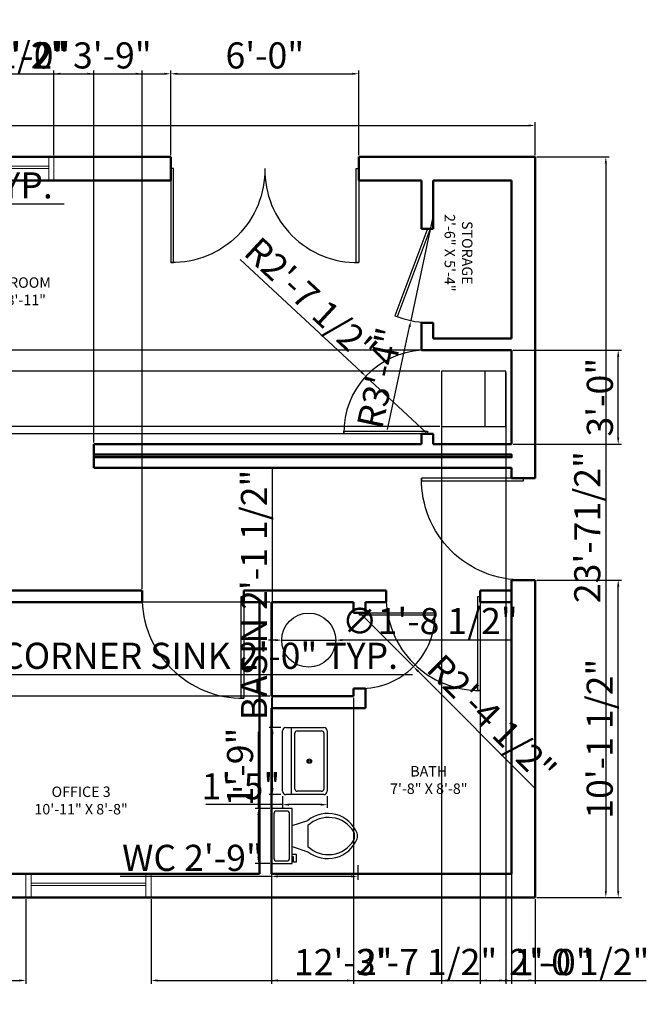
# Model space of a CAD drawing. Units: inches. Extents: x -53 to 650, y -41 to 348.
# Tile 3 of 3: x 410 to 650, y -41 to 336. Entities that reach past the tile are written whole.
import ezdxf

# ---------------------------------------------------------------- set-up
doc = ezdxf.new("R2010")
doc.units = ezdxf.units.IN
for name, color, linetype, lineweight in [('A-ANNO-DIMS', 2, 'Continuous', 18), ('A-AREA-IDEN', 7, 'Continuous', 25), ('A-DOOR', 3, 'Continuous', 25), ('A-EQPM', 8, 'Continuous', 25), ('A-FLOR-FIXT', 9, 'Continuous', 25), ('A-GLAZ', 4, 'Continuous', 18), ('A-WALL', 7, 'Continuous', 50), ('A-WALL-PATT', 7, 'Continuous', 13)]:
    doc.layers.add(name, color=color, linetype=linetype, lineweight=lineweight)
doc.styles.get("Standard").update_dxf_attribs({"font": 'arial.ttf'})
doc.dimstyles.new('ISO-25', dxfattribs={"dimtxt": 10, "dimasz": 2.5, "dimexe": 1.25, "dimexo": 0.625, "dimtad": 1, "dimlunit": 4, "dimtxsty": 'Standard', "dimcen": 2.5, "dimadec": 0, "dimazin": 0, "dimtfac": 1, "dimtmove": 0, "dimatfit": 3, "dimfxl": 1, "dimarcsym": 0})

# ---------------------------------------------------------------- blocks, each defined once
blk = doc.blocks.new('Sink-single - 30 in top')
blk.add_line((-15, -3.999996), (15, -3.999996))
for points in [[(-13.5, 0), (13.5, 0)], [(-15, -18.499996), (-15, -1.5)], [(15, -1.5), (15, -18.499996)], [(-13.5, -17.499996), (-13.5, -6.499996)], [(-12.5, -5.499996), (12.5, -5.499996)], [(13.5, -6.499996), (13.5, -17.499996)], [(13.5, -19.999996), (-13.5, -19.999996)], [(12.5, -18.499996), (-12.5, -18.499996)]]:
    blk.add_lwpolyline(points)
for radius in [1, 0.5]:
    blk.add_circle((0, -11.999996), radius)
for centre, radius, start, end in [((-13.5, -1.5), 1.5, 90, 180), ((13.5, -1.5), 1.5, 0, 90), ((-12.5, -6.499996), 1, 90, 180), ((12.5, -6.499996), 1, 0, 90), ((-12.5, -17.499996), 1, 180, 270), ((12.5, -17.499996), 1, 270, 0), ((-13.5, -18.499996), 1.5, 180, 270), ((13.5, -18.499996), 1.5, 270, 0)]:
    blk.add_arc(centre, radius, start, end)
blk = doc.blocks.new('Toilet - top')
for p, q in [((9.5, -6), (9.5, -2)), ((-10, -8.5), (-8, -8.5)), ((-10, -9.5), (-10, -8.5)), ((-7, -9.5), (-10, -9.5)), ((-8, -8.5), (-8, -8)), ((-7, -8), (-7, -9.5)), ((-4, -8), (-6, -14)), ((4, -8), (6, -14)), ((4, -14), (-4, -14))]:
    blk.add_line(p, q)
blk.add_lwpolyline([(10.5, -8), (10.5, 0), (-10.5, 0), (-10.5, -8)], close=True)
for points in [[(-9.5, -2), (-9.5, -6)], [(8.5, -1), (-8.5, -1)], [(-8.5, -7), (8.5, -7)]]:
    blk.add_lwpolyline(points)
for centre, radius, start, end in [((-8.62, -1.88), 0.884, 81.8699, 188.1301), ((8.62, -1.88), 0.884, 351.8699, 98.1301), ((-8.62, -6.12), 0.884, 171.8699, 278.1301), ((8.62, -6.12), 0.884, 261.8699, 8.1301), ((3.52, -21.58), 12.17, 141.4691, 247.9714), ((4.2, -21.82), 11.33, 136.3677, 238.9468), ((-3.52, -21.58), 12.17, 292.0284, 38.5307), ((-4.2, -21.82), 11.33, 301.053, 43.6321), ((0, -27.88), 4, 245.7318, 294.2682), ((0, -29), 4, 254.8605, 285.1395)]:
    blk.add_arc(centre, radius, start, end)
blk = doc.blocks.new('*D4')
at = {"layer": 'A-ANNO-DIMS', "color": 0, "lineweight": -2, "transparency": 16777216}
for p, q in [((0, 284.12), (0, 296.76)), ((2.5, 295.51), (604.5, 295.51)), ((607, 284.12), (607, 296.76))]:
    blk.add_line(p, q, dxfattribs=at)
at = {"layer": 'A-ANNO-DIMS', "color": 0, "transparency": 16777216}
for points in [[(2.5, 295.92), (2.5, 295.09), (0, 295.51)], [(604.5, 295.92), (604.5, 295.09), (607, 295.51)]]:
    blk.add_solid(points, dxfattribs=at)
at = {"layer": 'Defpoints', "color": 0, "transparency": 16777216}
for p in [(607, 295.51), (0, 283.5), (607, 283.5)]:
    blk.add_point(p, dxfattribs=at)
at = {"layer": 'A-ANNO-DIMS', "color": 0, "transparency": 16777216, "insert": (303.5, 301.24), "char_height": 10, "attachment_point": 5}
blk.add_mtext('50\'-0"', dxfattribs=at)
blk = doc.blocks.new('*D5')
at = {"layer": 'A-ANNO-DIMS', "color": 0, "lineweight": -2, "transparency": 16777216}
for p, q in [((607.63, 283.5), (635.31, 283.5)), ((634.06, 281), (634.06, 2.5)), ((607.63, 0), (635.31, 0))]:
    blk.add_line(p, q, dxfattribs=at)
at = {"layer": 'A-ANNO-DIMS', "color": 0, "transparency": 16777216}
for points in [[(633.65, 281), (634.48, 281), (634.06, 283.5)], [(633.65, 2.5), (634.48, 2.5), (634.06, 0)]]:
    blk.add_solid(points, dxfattribs=at)
at = {"layer": 'Defpoints', "color": 0, "transparency": 16777216}
for p in [(607, 283.5), (607, 0), (634.06, 0)]:
    blk.add_point(p, dxfattribs=at)
at = {"layer": 'A-ANNO-DIMS', "color": 0, "transparency": 16777216, "insert": (628.26, 141.75), "char_height": 10, "attachment_point": 5, "rotation": 90}
blk.add_mtext('23\'-71/2"', dxfattribs=at)
blk = doc.blocks.new('DOOR-SWING-39IN')
for p, q in [((38, 0), (38, 39)), ((38, 39), (39, 39)), ((39, 39), (39, 0)), ((39, 0), (38, 0))]:
    blk.add_line(p, q)
blk.add_arc((38.5, 38.5), 38.5, 179.2559, 270.7441)
blk = doc.blocks.new('DOOR-SWING-36IN')
for p, q in [((35.001, 0.001), (35.001, 36.001)), ((35.001, 36.001), (36.001, 36.001)), ((36.001, 36.001), (36.001, 0.001)), ((36.001, 0.001), (35.001, 0.001))]:
    blk.add_line(p, q)
blk.add_arc((35.501, 35.501), 35.504, 179.19307, 270.80693)
blk = doc.blocks.new('WIN-48IN')
for p, q in [((0, 9), (0, 0)), ((2, 0), (2, 9)), ((46, 0), (46, 9)), ((48, 9), (48, 0)), ((2, 5.5), (46, 5.5)), ((2, 4.5), (46, 4.5))]:
    blk.add_line(p, q)
blk.add_lwpolyline([(48, 9), (0, 9), (0, 0), (48, 0)], close=True)
blk = doc.blocks.new('WIN-60IN')
for p, q in [((0, 9), (0, 0)), ((2, 0), (2, 9)), ((58, 0), (58, 9)), ((60, 9), (60, 0)), ((2, 5.5), (58, 5.5)), ((2, 4.5), (58, 4.5))]:
    blk.add_line(p, q)
blk.add_lwpolyline([(60, 9), (0, 9), (0, 0), (60, 0)], close=True)
blk = doc.blocks.new('*D17')
at = {"layer": 'A-ANNO-DIMS', "color": 0, "lineweight": -2, "transparency": 16777216}
for p, q in [((211.5, 273.88), (211.5, 264.25)), ((271.5, 273.88), (271.5, 264.25)), ((214, 265.5), (269, 265.5)), ((271.5, 265.5), (426.63, 265.5))]:
    blk.add_line(p, q, dxfattribs=at)
at = {"layer": 'A-ANNO-DIMS', "color": 0, "transparency": 16777216}
for points in [[(214, 265.92), (214, 265.08), (211.5, 265.5)], [(269, 265.92), (269, 265.08), (271.5, 265.5)]]:
    blk.add_solid(points, dxfattribs=at)
at = {"layer": 'Defpoints', "color": 0, "transparency": 16777216}
for p in [(211.5, 274.5), (271.5, 274.5), (271.5, 265.5)]:
    blk.add_point(p, dxfattribs=at)
at = {"layer": 'A-ANNO-DIMS', "color": 0, "transparency": 16777216, "insert": (350.31, 271.3), "char_height": 10, "attachment_point": 5}
blk.add_mtext('WINDOW W2 5\'-0" TYP.', dxfattribs=at)
blk = doc.blocks.new('*D19')
at = {"layer": 'A-ANNO-DIMS', "color": 0, "lineweight": -2, "transparency": 16777216}
for p, q in [((370.5, 88.37), (370.5, 84.15)), ((394.5, 88.37), (394.5, 84.15)), ((373, 85.4), (392, 85.4)), ((394.5, 85.4), (560, 85.4))]:
    blk.add_line(p, q, dxfattribs=at)
at = {"layer": 'A-ANNO-DIMS', "color": 0, "transparency": 16777216}
for points in [[(373, 85.82), (373, 84.98), (370.5, 85.4)], [(392, 85.82), (392, 84.98), (394.5, 85.4)]]:
    blk.add_solid(points, dxfattribs=at)
at = {"layer": 'Defpoints', "color": 0, "transparency": 16777216}
for p in [(370.5, 89), (394.5, 89), (394.5, 85.4)]:
    blk.add_point(p, dxfattribs=at)
at = {"layer": 'A-ANNO-DIMS', "color": 0, "transparency": 16777216, "insert": (478.5, 91.2), "char_height": 10, "attachment_point": 5}
blk.add_mtext('CORNER SINK 2\'-0" TYP.', dxfattribs=at)
blk = doc.blocks.new('*D23')
at = {"layer": 'A-ANNO-DIMS', "color": 0, "lineweight": -2, "transparency": 16777216}
for p, q in [((506.45, 65.01), (506.45, 164.01)), ((509.67, 65.01), (505.2, 65.01)), ((506.45, 41.86), (506.45, 62.51)), ((509.67, 39.36), (505.2, 39.36))]:
    blk.add_line(p, q, dxfattribs=at)
at = {"layer": 'A-ANNO-DIMS', "color": 0, "transparency": 16777216}
for points in [[(506.03, 62.51), (506.86, 62.51), (506.45, 65.01)], [(506.03, 41.86), (506.86, 41.86), (506.45, 39.36)]]:
    blk.add_solid(points, dxfattribs=at)
at = {"layer": 'Defpoints', "color": 0, "transparency": 16777216}
for p in [(506.45, 65.01), (510.3, 65.01), (510.3, 39.36)]:
    blk.add_point(p, dxfattribs=at)
at = {"layer": 'A-ANNO-DIMS', "color": 0, "transparency": 16777216, "insert": (500.65, 115.76), "char_height": 10, "attachment_point": 5, "rotation": 90}
blk.add_mtext('BASIN 2\'-1 1/2"', dxfattribs=at)
blk = doc.blocks.new('*D24')
at = {"layer": 'A-ANNO-DIMS', "color": 0, "lineweight": -2, "transparency": 16777216}
for p, q in [((510.3, 38.73), (510.3, 34.26)), ((527.4, 38.73), (527.4, 34.26)), ((510.3, 35.51), (480.9, 35.51)), ((524.9, 35.51), (512.8, 35.51))]:
    blk.add_line(p, q, dxfattribs=at)
at = {"layer": 'A-ANNO-DIMS', "color": 0, "transparency": 16777216}
for points in [[(512.8, 35.93), (512.8, 35.09), (510.3, 35.51)], [(524.9, 35.93), (524.9, 35.09), (527.4, 35.51)]]:
    blk.add_solid(points, dxfattribs=at)
at = {"layer": 'Defpoints', "color": 0, "transparency": 16777216}
for p in [(510.3, 39.36), (527.4, 39.36), (510.3, 35.51)]:
    blk.add_point(p, dxfattribs=at)
at = {"layer": 'A-ANNO-DIMS', "color": 0, "transparency": 16777216, "insert": (494.35, 41.24), "char_height": 10, "attachment_point": 5}
blk.add_mtext('1\'-5"', dxfattribs=at)
blk = doc.blocks.new('*D25')
at = {"layer": 'A-ANNO-DIMS', "color": 0, "lineweight": -2, "transparency": 16777216}
for p, q in [((506, 12.38), (506, 6.79)), ((539.05, 12.38), (539.05, 6.79)), ((506, 8.04), (448.1, 8.04)), ((536.55, 8.04), (508.5, 8.04))]:
    blk.add_line(p, q, dxfattribs=at)
at = {"layer": 'A-ANNO-DIMS', "color": 0, "transparency": 16777216}
for points in [[(508.5, 8.46), (508.5, 7.63), (506, 8.04)], [(536.55, 8.46), (536.55, 7.63), (539.05, 8.04)]]:
    blk.add_solid(points, dxfattribs=at)
at = {"layer": 'Defpoints', "color": 0, "transparency": 16777216}
for p in [(506, 13), (539.05, 13), (506, 8.04)]:
    blk.add_point(p, dxfattribs=at)
at = {"layer": 'A-ANNO-DIMS', "color": 0, "transparency": 16777216, "insert": (475.8, 13.84), "char_height": 10, "attachment_point": 5}
blk.add_mtext('WC 2\'-9"', dxfattribs=at)
blk = doc.blocks.new('*D26')
at = {"layer": 'A-ANNO-DIMS', "color": 0, "lineweight": -2, "transparency": 16777216}
for p, q in [((501.04, 34), (501.04, 63.39)), ((505.38, 34), (499.79, 34)), ((501.04, 15.5), (501.04, 31.5)), ((505.38, 13), (499.79, 13))]:
    blk.add_line(p, q, dxfattribs=at)
at = {"layer": 'A-ANNO-DIMS', "color": 0, "transparency": 16777216}
for points in [[(500.63, 31.5), (501.46, 31.5), (501.04, 34)], [(500.63, 15.5), (501.46, 15.5), (501.04, 13)]]:
    blk.add_solid(points, dxfattribs=at)
at = {"layer": 'Defpoints', "color": 0, "transparency": 16777216}
for p in [(501.04, 34), (506, 34), (506, 13)]:
    blk.add_point(p, dxfattribs=at)
at = {"layer": 'A-ANNO-DIMS', "color": 0, "transparency": 16777216, "insert": (495.31, 49.95), "char_height": 10, "attachment_point": 5, "rotation": 90}
blk.add_mtext('1\'-9"', dxfattribs=at)
blk = doc.blocks.new('*D30')
at = {"layer": 'A-ANNO-DIMS', "color": 0, "lineweight": -2, "transparency": 16777216}
for p, q in [((422.75, 284.12), (422.75, 316.56)), ((425.25, 315.31), (465, 315.31)), ((467.5, 284.12), (467.5, 316.56))]:
    blk.add_line(p, q, dxfattribs=at)
at = {"layer": 'A-ANNO-DIMS', "color": 0, "transparency": 16777216}
for points in [[(425.25, 315.72), (425.25, 314.89), (422.75, 315.31)], [(465, 315.72), (465, 314.89), (467.5, 315.31)]]:
    blk.add_solid(points, dxfattribs=at)
at = {"layer": 'Defpoints', "color": 0, "transparency": 16777216}
for p in [(467.5, 315.31), (422.75, 283.5), (467.5, 283.5)]:
    blk.add_point(p, dxfattribs=at)
at = {"layer": 'A-ANNO-DIMS', "color": 0, "transparency": 16777216, "insert": (445.12, 321.04), "char_height": 10, "attachment_point": 5}
blk.add_mtext('3\'-9"', dxfattribs=at)
blk = doc.blocks.new('*D31')
at = {"layer": 'A-ANNO-DIMS', "color": 0, "lineweight": -2, "transparency": 16777216}
for p, q in [((467.5, 284.12), (467.5, 316.56)), ((470, 315.31), (537, 315.31)), ((539.5, 284.12), (539.5, 316.56))]:
    blk.add_line(p, q, dxfattribs=at)
at = {"layer": 'A-ANNO-DIMS', "color": 0, "transparency": 16777216}
for points in [[(470, 315.72), (470, 314.89), (467.5, 315.31)], [(537, 315.72), (537, 314.89), (539.5, 315.31)]]:
    blk.add_solid(points, dxfattribs=at)
at = {"layer": 'Defpoints', "color": 0, "transparency": 16777216}
for p in [(539.5, 315.31), (467.5, 283.5), (539.5, 283.5)]:
    blk.add_point(p, dxfattribs=at)
at = {"layer": 'A-ANNO-DIMS', "color": 0, "transparency": 16777216, "insert": (503.5, 321.04), "char_height": 10, "attachment_point": 5}
blk.add_mtext('6\'-0"', dxfattribs=at)
blk = doc.blocks.new('*D34')
at = {"layer": 'A-ANNO-DIMS', "color": 0, "lineweight": -2, "transparency": 16777216}
for p, q in [((223, -0.62), (223, -33.05)), ((412, -0.62), (412, -33.05)), ((225.5, -31.8), (409.5, -31.8))]:
    blk.add_line(p, q, dxfattribs=at)
at = {"layer": 'A-ANNO-DIMS', "color": 0, "transparency": 16777216}
for points in [[(225.5, -31.39), (225.5, -32.22), (223, -31.8)], [(409.5, -31.39), (409.5, -32.22), (412, -31.8)]]:
    blk.add_solid(points, dxfattribs=at)
at = {"layer": 'Defpoints', "color": 0, "transparency": 16777216}
for p in [(223, 0), (412, 0), (412, -31.8)]:
    blk.add_point(p, dxfattribs=at)
at = {"layer": 'A-ANNO-DIMS', "color": 0, "transparency": 16777216, "insert": (317.5, -26.07), "char_height": 10, "attachment_point": 5}
blk.add_mtext('15\'-9"', dxfattribs=at)
blk = doc.blocks.new('*D35')
at = {"layer": 'A-ANNO-DIMS', "color": 0, "lineweight": -2, "transparency": 16777216}
for p, q in [((460, -0.62), (460, -33.05)), ((607, -0.62), (607, -33.05)), ((462.5, -31.8), (604.5, -31.8))]:
    blk.add_line(p, q, dxfattribs=at)
at = {"layer": 'A-ANNO-DIMS', "color": 0, "transparency": 16777216}
for points in [[(462.5, -31.39), (462.5, -32.22), (460, -31.8)], [(604.5, -31.39), (604.5, -32.22), (607, -31.8)]]:
    blk.add_solid(points, dxfattribs=at)
at = {"layer": 'Defpoints', "color": 0, "transparency": 16777216}
for p in [(460, 0), (607, 0), (607, -31.8)]:
    blk.add_point(p, dxfattribs=at)
at = {"layer": 'A-ANNO-DIMS', "color": 0, "transparency": 16777216, "insert": (533.5, -26.07), "char_height": 10, "attachment_point": 5}
blk.add_mtext('12\'-3"', dxfattribs=at)
blk = doc.blocks.new('*D36')
at = {"layer": 'A-ANNO-DIMS', "color": 0, "lineweight": -2, "transparency": 16777216}
for p, q in [((607.63, 121.5), (640.06, 121.5)), ((638.81, 2.5), (638.81, 119)), ((607.63, 0), (640.06, 0))]:
    blk.add_line(p, q, dxfattribs=at)
at = {"layer": 'A-ANNO-DIMS', "color": 0, "transparency": 16777216}
for points in [[(638.39, 119), (639.22, 119), (638.81, 121.5)], [(638.39, 2.5), (639.22, 2.5), (638.81, 0)]]:
    blk.add_solid(points, dxfattribs=at)
at = {"layer": 'Defpoints', "color": 0, "transparency": 16777216}
for p in [(607, 121.5), (638.81, 121.5), (607, 0)]:
    blk.add_point(p, dxfattribs=at)
at = {"layer": 'A-ANNO-DIMS', "color": 0, "transparency": 16777216, "insert": (633.01, 60.75), "char_height": 10, "attachment_point": 5, "rotation": 90}
blk.add_mtext('10\'-1 1/2"', dxfattribs=at)
blk = doc.blocks.new('*D38')
at = {"layer": 'A-ANNO-DIMS', "color": 0, "lineweight": -2, "transparency": 16777216}
for p, q in [((390, 174.12), (390, 316.56)), ((392.5, 315.31), (435.5, 315.31)), ((438, 174.12), (438, 316.56))]:
    blk.add_line(p, q, dxfattribs=at)
at = {"layer": 'A-ANNO-DIMS', "color": 0, "transparency": 16777216}
for points in [[(392.5, 315.72), (392.5, 314.89), (390, 315.31)], [(435.5, 315.72), (435.5, 314.89), (438, 315.31)]]:
    blk.add_solid(points, dxfattribs=at)
at = {"layer": 'Defpoints', "color": 0, "transparency": 16777216}
for p in [(438, 315.31), (390, 173.5), (438, 173.5)]:
    blk.add_point(p, dxfattribs=at)
at = {"layer": 'A-ANNO-DIMS', "color": 0, "transparency": 16777216, "insert": (414, 321.04), "char_height": 10, "attachment_point": 5}
blk.add_mtext('4\'-0"', dxfattribs=at)
blk = doc.blocks.new('*D41')
at = {"layer": 'A-ANNO-DIMS', "color": 0, "lineweight": -2, "transparency": 16777216}
for p, q in [((598.63, 209.5), (640.06, 209.5)), ((638.81, 176), (638.81, 207)), ((598.63, 173.5), (640.06, 173.5))]:
    blk.add_line(p, q, dxfattribs=at)
at = {"layer": 'A-ANNO-DIMS', "color": 0, "transparency": 16777216}
for points in [[(638.39, 207), (639.22, 207), (638.81, 209.5)], [(638.39, 176), (639.22, 176), (638.81, 173.5)]]:
    blk.add_solid(points, dxfattribs=at)
at = {"layer": 'Defpoints', "color": 0, "transparency": 16777216}
for p in [(598, 209.5), (638.81, 209.5), (598, 173.5)]:
    blk.add_point(p, dxfattribs=at)
at = {"layer": 'A-ANNO-DIMS', "color": 0, "transparency": 16777216, "insert": (633.07, 191.5), "char_height": 10, "attachment_point": 5, "rotation": 90}
blk.add_mtext('3\'-0"', dxfattribs=at)
blk = doc.blocks.new('*D42')
at = {"layer": 'A-ANNO-DIMS', "color": 0, "lineweight": -2, "transparency": 16777216}
for p, q in [((506, 76.38), (506, -33.06)), ((537.5, 76.38), (537.5, -33.06)), ((508.5, -31.8), (535, -31.8)), ((537.5, -31.8), (591.3, -31.8))]:
    blk.add_line(p, q, dxfattribs=at)
at = {"layer": 'A-ANNO-DIMS', "color": 0, "transparency": 16777216}
for points in [[(508.5, -31.39), (508.5, -32.22), (506, -31.8)], [(535, -31.39), (535, -32.22), (537.5, -31.8)]]:
    blk.add_solid(points, dxfattribs=at)
at = {"layer": 'Defpoints', "color": 0, "transparency": 16777216}
for p in [(506, 77), (537.5, 77), (537.5, -31.8)]:
    blk.add_point(p, dxfattribs=at)
at = {"layer": 'A-ANNO-DIMS', "color": 0, "transparency": 16777216, "insert": (565.65, -26.01), "char_height": 10, "attachment_point": 5}
blk.add_mtext('2\'-7 1/2"', dxfattribs=at)
blk = doc.blocks.new('*D43')
at = {"layer": 'A-ANNO-DIMS', "color": 0, "lineweight": -2, "transparency": 16777216}
for p, q in [((505.38, 113), (-33.05, 113)), ((-31.81, 79.5), (-31.81, 110.5)), ((505.38, 77), (-33.05, 77))]:
    blk.add_line(p, q, dxfattribs=at)
at = {"layer": 'A-ANNO-DIMS', "color": 0, "transparency": 16777216}
for points in [[(-32.22, 110.5), (-31.39, 110.5), (-31.81, 113)], [(-32.22, 79.5), (-31.39, 79.5), (-31.81, 77)]]:
    blk.add_solid(points, dxfattribs=at)
at = {"layer": 'Defpoints', "color": 0, "transparency": 16777216}
for p in [(-31.81, 113), (506, 113), (506, 77)]:
    blk.add_point(p, dxfattribs=at)
at = {"layer": 'A-ANNO-DIMS', "color": 0, "transparency": 16777216, "insert": (-37.54, 95), "char_height": 10, "attachment_point": 5, "rotation": 90}
blk.add_mtext('3\'-0"', dxfattribs=at)
blk = doc.blocks.new('*D46')
at = {"layer": 'A-ANNO-DIMS', "color": 0, "lineweight": -2, "transparency": 16777216}
for p, q in [((370.5, 118.12), (370.5, 316.56)), ((373, 315.31), (454, 315.31)), ((456.5, 118.12), (456.5, 316.56))]:
    blk.add_line(p, q, dxfattribs=at)
at = {"layer": 'A-ANNO-DIMS', "color": 0, "transparency": 16777216}
for points in [[(373, 315.72), (373, 314.89), (370.5, 315.31)], [(454, 315.72), (454, 314.89), (456.5, 315.31)]]:
    blk.add_solid(points, dxfattribs=at)
at = {"layer": 'Defpoints', "color": 0, "transparency": 16777216}
for p in [(456.5, 315.31), (370.5, 117.5), (456.5, 117.5)]:
    blk.add_point(p, dxfattribs=at)
at = {"layer": 'A-ANNO-DIMS', "color": 0, "transparency": 16777216, "insert": (413.5, 320.95), "char_height": 10, "attachment_point": 5}
blk.add_mtext('7\'-2"', dxfattribs=at)
blk = doc.blocks.new('*D47')
at = {"layer": 'A-ANNO-DIMS', "color": 0, "lineweight": -2, "transparency": 16777216}
for p, q in [((586, 112.38), (586, -33.06)), ((598, 112.38), (598, -33.06)), ((588.5, -31.8), (595.5, -31.8)), ((598, -31.8), (627.39, -31.8))]:
    blk.add_line(p, q, dxfattribs=at)
at = {"layer": 'A-ANNO-DIMS', "color": 0, "transparency": 16777216}
for points in [[(588.5, -31.39), (588.5, -32.22), (586, -31.8)], [(595.5, -31.39), (595.5, -32.22), (598, -31.8)]]:
    blk.add_solid(points, dxfattribs=at)
at = {"layer": 'Defpoints', "color": 0, "transparency": 16777216}
for p in [(586, 113), (598, 113), (598, -31.8)]:
    blk.add_point(p, dxfattribs=at)
at = {"layer": 'A-ANNO-DIMS', "color": 0, "transparency": 16777216, "insert": (613.95, -26.07), "char_height": 10, "attachment_point": 5}
blk.add_mtext('1\'-0"', dxfattribs=at)
blk = doc.blocks.new('*D52')
at = {"layer": 'A-ANNO-DIMS', "color": 0, "lineweight": -2, "transparency": 16777216}
for p, q in [((562.88, 209.5), (-33.06, 209.5)), ((-31.81, 180), (-31.81, 207)), ((562.88, 177.5), (-33.06, 177.5))]:
    blk.add_line(p, q, dxfattribs=at)
at = {"layer": 'A-ANNO-DIMS', "color": 0, "transparency": 16777216}
for points in [[(-32.22, 207), (-31.39, 207), (-31.81, 209.5)], [(-32.22, 180), (-31.39, 180), (-31.81, 177.5)]]:
    blk.add_solid(points, dxfattribs=at)
at = {"layer": 'Defpoints', "color": 0, "transparency": 16777216}
for p in [(-31.81, 209.5), (563.5, 209.5), (563.5, 177.5)]:
    blk.add_point(p, dxfattribs=at)
at = {"layer": 'A-ANNO-DIMS', "color": 0, "transparency": 16777216, "insert": (-37.54, 193.5), "char_height": 10, "attachment_point": 5, "rotation": 90}
blk.add_mtext('2\'-8"', dxfattribs=at)
blk = doc.blocks.new('*D53')
at = {"layer": 'A-ANNO-DIMS', "color": 0, "lineweight": -2, "transparency": 16777216}
for p, q in [((363.5, 315.31), (361, 315.31)), ((366, 118.12), (366, 316.56)), ((366, 315.31), (370.5, 315.31)), ((370.5, 118.12), (370.5, 316.56)), ((373, 315.31), (426.63, 315.31))]:
    blk.add_line(p, q, dxfattribs=at)
at = {"layer": 'A-ANNO-DIMS', "color": 0, "transparency": 16777216}
for points in [[(363.5, 315.72), (363.5, 314.89), (366, 315.31)], [(373, 315.72), (373, 314.89), (370.5, 315.31)]]:
    blk.add_solid(points, dxfattribs=at)
at = {"layer": 'Defpoints', "color": 0, "transparency": 16777216}
for p in [(370.5, 315.31), (366, 117.5), (370.5, 117.5)]:
    blk.add_point(p, dxfattribs=at)
at = {"layer": 'A-ANNO-DIMS', "color": 0, "transparency": 16777216, "insert": (401.07, 321.1), "char_height": 10, "attachment_point": 5}
blk.add_mtext('0\'-4 1/2"', dxfattribs=at)
blk = doc.blocks.new('*D55')
at = {"layer": 'A-ANNO-DIMS', "color": 0, "lineweight": -2, "transparency": 16777216}
for p, q in [((571.1, 200.8), (571.1, -33.06)), ((595.76, 200.8), (595.76, -33.06)), ((573.6, -31.8), (593.26, -31.8)), ((595.76, -31.8), (649.56, -31.8))]:
    blk.add_line(p, q, dxfattribs=at)
at = {"layer": 'A-ANNO-DIMS', "color": 0, "transparency": 16777216}
for points in [[(573.6, -31.39), (573.6, -32.22), (571.1, -31.8)], [(593.26, -31.39), (593.26, -32.22), (595.76, -31.8)]]:
    blk.add_solid(points, dxfattribs=at)
at = {"layer": 'Defpoints', "color": 0, "transparency": 16777216}
for p in [(571.1, 201.42), (595.76, 201.42), (595.76, -31.8)]:
    blk.add_point(p, dxfattribs=at)
at = {"layer": 'A-ANNO-DIMS', "color": 0, "transparency": 16777216, "insert": (623.91, -26.01), "char_height": 10, "attachment_point": 5}
blk.add_mtext('2\'-0 1/2"', dxfattribs=at)
blk = doc.blocks.new('*D56')
at = {"layer": 'A-ANNO-DIMS', "color": 0, "lineweight": -2, "transparency": 16777216}
for p, q in [((-31.81, 201.42), (-31.81, 230.81)), ((570.47, 201.42), (-33.05, 201.42)), ((-31.81, 182.73), (-31.81, 198.92)), ((570.47, 180.23), (-33.05, 180.23))]:
    blk.add_line(p, q, dxfattribs=at)
at = {"layer": 'A-ANNO-DIMS', "color": 0, "transparency": 16777216}
for points in [[(-32.22, 198.92), (-31.39, 198.92), (-31.81, 201.42)], [(-32.22, 182.73), (-31.39, 182.73), (-31.81, 180.23)]]:
    blk.add_solid(points, dxfattribs=at)
at = {"layer": 'Defpoints', "color": 0, "transparency": 16777216}
for p in [(-31.81, 201.42), (571.1, 201.42), (571.1, 180.23)]:
    blk.add_point(p, dxfattribs=at)
at = {"layer": 'A-ANNO-DIMS', "color": 0, "transparency": 16777216, "insert": (-37.54, 217.37), "char_height": 10, "attachment_point": 5, "rotation": 90}
blk.add_mtext('1\'-9"', dxfattribs=at)
blk = doc.blocks.new('*D57')
at = {"layer": 'A-ANNO-DIMS', "color": 0, "lineweight": -2, "transparency": 16777216}
for p, q in [((507.47, 98.49), (504.97, 98.49)), ((509.97, 98.49), (530.67, 98.49)), ((597.68, 98.49), (533.17, 98.49))]:
    blk.add_line(p, q, dxfattribs=at)
at = {"layer": 'A-ANNO-DIMS', "color": 0, "transparency": 16777216}
for points in [[(507.47, 98.91), (507.47, 98.07), (509.97, 98.49)], [(533.17, 98.91), (533.17, 98.07), (530.67, 98.49)]]:
    blk.add_solid(points, dxfattribs=at)
at = {"layer": 'Defpoints', "color": 0, "transparency": 16777216}
for p in [(509.97, 98.49), (530.67, 98.49)]:
    blk.add_point(p, dxfattribs=at)
at = {"layer": 'A-ANNO-DIMS', "color": 0, "transparency": 16777216, "insert": (566.68, 104.5), "char_height": 10, "attachment_point": 5, "rotation": 359.9997}
blk.add_mtext('∅1\'-8 1/2"', dxfattribs=at)
blk = doc.blocks.new('*D58')
at = {"layer": 'A-ANNO-DIMS', "color": 0, "lineweight": -2, "transparency": 16777216}
for p, q in [((567.75, 259.91), (559.41, 220.83)), ((550.52, 179.09), (558.89, 218.38))]:
    blk.add_line(p, q, dxfattribs=at)
at = {"layer": 'A-ANNO-DIMS', "color": 0, "transparency": 16777216}
blk.add_solid([(558.49, 218.47), (559.3, 218.3), (559.41, 220.83)], dxfattribs=at)
at = {"layer": 'Defpoints', "color": 0, "transparency": 16777216}
for p in [(567.75, 259.91), (559.41, 220.83)]:
    blk.add_point(p, dxfattribs=at)
at = {"layer": 'A-ANNO-DIMS', "color": 0, "transparency": 16777216, "insert": (548.81, 198.57), "char_height": 10, "attachment_point": 5, "rotation": 77.9667}
blk.add_mtext('R3\'-4"', dxfattribs=at)
blk = doc.blocks.new('*D59')
at = {"layer": 'A-ANNO-DIMS', "color": 0, "lineweight": -2, "transparency": 16777216}
for p, q in [((540.25, 108.5), (560.41, 88.34)), ((606.87, 41.88), (562.17, 86.58))]:
    blk.add_line(p, q, dxfattribs=at)
at = {"layer": 'A-ANNO-DIMS', "color": 0, "transparency": 16777216}
blk.add_solid([(562.47, 86.87), (561.88, 86.28), (560.41, 88.34)], dxfattribs=at)
at = {"layer": 'Defpoints', "color": 0, "transparency": 16777216}
for p in [(540.25, 108.5), (560.41, 88.34)]:
    blk.add_point(p, dxfattribs=at)
at = {"layer": 'A-ANNO-DIMS', "color": 0, "transparency": 16777216, "insert": (589.5, 67.44), "char_height": 10, "attachment_point": 5, "rotation": 315}
blk.add_mtext('R2\'-4 1/2"', dxfattribs=at)
blk = doc.blocks.new('*D61')
at = {"layer": 'A-ANNO-DIMS', "color": 0, "lineweight": -2, "transparency": 16777216}
for p, q in [((494.07, 244.22), (540.36, 201.19)), ((565.3, 178), (542.19, 199.48))]:
    blk.add_line(p, q, dxfattribs=at)
at = {"layer": 'A-ANNO-DIMS', "color": 0, "transparency": 16777216}
blk.add_solid([(540.64, 201.49), (540.08, 200.88), (542.19, 199.48)], dxfattribs=at)
at = {"layer": 'Defpoints', "color": 0, "transparency": 16777216}
for p in [(542.19, 199.48), (565.3, 178)]:
    blk.add_point(p, dxfattribs=at)
at = {"layer": 'A-ANNO-DIMS', "color": 0, "transparency": 16777216, "insert": (520.24, 227.8), "char_height": 10, "attachment_point": 5, "rotation": 317.0862}
blk.add_mtext('R2\'-7 1/2"', dxfattribs=at)

msp = doc.modelspace()

# ---------------------------------------------------------------- hatches: boundary and pattern name
at = {"layer": 'A-WALL-PATT'}
h = msp.add_hatch(color=256, dxfattribs=at)
h.dxf.hatch_style = 1
h.paths.add_polyline_path([(9, 169.5), (9, 168.5), (122, 168.5), (122, 169, -0.0032466), (121.997, 169.5)])
h.paths.add_polyline_path([(161, 169.5), (161, 168.5), (181.5, 168.5), (181.5, 169.5)])
h.paths.add_polyline_path([(220.503, 169.5), (220.503, 168.5), (390, 168.5), (390, 169.5)])
h.paths.add_polyline_path([(598, 168.5), (598, 169.5), (438, 169.5), (438, 168.5)])

# ---------------------------------------------------------------- linework, layer by layer
at = {"layer": 'A-DOOR'}
for p, q in [((565.881, 256.35), (553.291, 222.656)), ((566.818, 256), (554.228, 222.306)), ((533.75, 177.5), (533.75, 178.5)), ((533.75, 178.5), (565.75, 178.5)), ((565.75, 177.5), (533.75, 177.5)), ((565.75, 178.5), (565.75, 177.5)), ((539.75, 109), (568.75, 109)), ((539.75, 108), (539.75, 109)), ((568.75, 108), (539.75, 108)), ((568.75, 109), (568.75, 108))]:
    msp.add_line(p, q, dxfattribs=at)
for centre, radius, start, end in [((567.745, 259.911), 39.961, 248.79506, 267.13818), ((565.297, 178), 31.551, 93.26554, 180.90802), ((540.25, 108.5), 28.504, 268.99491, 1.00509)]:
    msp.add_arc(centre, radius, start, end, dxfattribs=at)
at = {"layer": 'A-EQPM'}
for p, q in [((595.759, 201.421), (571.095, 201.421)), ((571.095, 201.421), (571.095, 180.228)), ((587.867, 180.228), (587.867, 201.421)), ((595.759, 180.228), (595.759, 201.421)), ((571.095, 180.228), (595.759, 180.228))]:
    msp.add_line(p, q, dxfattribs=at)
msp.add_circle((520.317, 98.491), 10.351, dxfattribs=at)
at = {"layer": 'A-WALL'}
for p, q in [((123, 283.5), (467.5, 283.5)), ((467.5, 283.5), (467.5, 274.5)), ((539.5, 283.5), (539.5, 274.5)), ((539.5, 283.5), (607, 283.5)), ((607, 283.5), (607, 160.5)), ((318, 274.5), (467.5, 274.5)), ((539.5, 274.5), (563.5, 274.5)), ((563.5, 274.5), (563.5, 256)), ((568, 274.5), (568, 256)), ((568, 274.5), (598, 274.5)), ((598, 274.5), (598, 214)), ((563.5, 256), (568, 256)), ((563.5, 220), (568, 220)), ((563.5, 220), (563.5, 209.5)), ((568, 220), (568, 214)), ((568, 214), (598, 214)), ((563.5, 209.5), (598, 209.5)), ((598, 209.5), (598, 173.5)), ((563.5, 177.5), (568, 177.5)), ((563.5, 177.5), (563.5, 173.5)), ((568, 177.5), (568, 173.5)), ((438, 173.5), (438, 164.5)), ((438, 173.5), (563.5, 173.5)), ((568, 173.5), (598, 173.5)), ((438, 169.5), (598, 169.5)), ((438, 168.5), (598, 168.5)), ((598, 169.5), (598, 168.5)), ((438, 164.5), (598, 164.5)), ((598, 164.5), (598, 160.5)), ((598, 160.5), (607, 160.5)), ((598, 121.5), (607, 121.5)), ((598, 121.5), (598, 9)), ((607, 121.5), (607, 0)), ((314, 117.5), (456.5, 117.5)), ((456.5, 117.5), (456.5, 113)), ((495.5, 117.5), (495.5, 113)), ((495.5, 117.5), (550, 117.5)), ((550, 117.5), (550, 113)), ((586, 117.5), (586, 113)), ((586, 117.5), (598, 117.5)), ((314, 113), (456.5, 113)), ((495.5, 113), (501.5, 113)), ((501.5, 113), (501.5, 9)), ((506, 113), (506, 77)), ((506, 113), (537.5, 113)), ((537.5, 113), (537.5, 109)), ((542, 113), (542, 109)), ((542, 113), (550, 113)), ((586, 113), (598, 113)), ((537.5, 109), (542, 109)), ((537.5, 80), (542, 80)), ((537.5, 80), (537.5, 77)), ((542, 80), (542, 72.5)), ((506, 77), (537.5, 77)), ((506, 72.5), (542, 72.5)), ((506, 72.5), (506, 9)), ((370.5, 9), (501.5, 9)), ((506, 9), (598, 9)), ((93, 0), (607, 0))]:
    msp.add_line(p, q, dxfattribs=at)
msp.add_lwpolyline([(438, 169.5), (598, 169.5), (598, 168.5), (438, 168.5)], close=True, dxfattribs=at)

# ---------------------------------------------------------------- block references
at = {"layer": 'A-DOOR', "extrusion": (0, 0, -1), "zscale": -1}
msp.add_blockref('DOOR-SWING-36IN', (-503.501, 242.999), dxfattribs=at)
at = {"layer": 'A-DOOR'}
for name, p in [('DOOR-SWING-36IN', (503.499, 242.999)), ('DOOR-SWING-39IN', (456.5, 76.25)), ('DOOR-SWING-36IN', (549.999, 79.249))]:
    msp.add_blockref(name, p, dxfattribs=at)
at = {"layer": 'A-DOOR', "extrusion": (0, 0, -1), "zscale": -1, "rotation": 90.00000000000003}
msp.add_blockref('DOOR-SWING-39IN', (-563.5, 121.5), dxfattribs=at)
at = {"layer": 'A-FLOR-FIXT', "xscale": 0.8551398701562579, "yscale": 0.8551398701562579, "zscale": 0.8551398701562579, "rotation": 90}
msp.add_blockref('Sink-single - 30 in top', (510.295, 52.185), dxfattribs=at)
at = {"layer": 'A-FLOR-FIXT', "rotation": 90}
msp.add_blockref('Toilet - top', (506, 23.5), dxfattribs=at)
at = {"layer": 'A-GLAZ'}
for name, p in [('WIN-60IN', (362.75, 274.5)), ('WIN-48IN', (412, 0))]:
    msp.add_blockref(name, p, dxfattribs=at)

# ---------------------------------------------------------------- texts
at = {"layer": 'A-AREA-IDEN', "insert": (583, 279.531), "char_height": 4, "attachment_point": 1, "rotation": 270}
msp.add_mtext_dynamic_manual_height_columns('\\pxqc;STORAGE\\P2\'-6" X 5\'-4"', width=65.53067, gutter_width=12.5, heights=[0], dxfattribs=at)
at = {"layer": 'A-AREA-IDEN', "char_height": 4, "attachment_point": 1}
for s, insert in [('\\pxqc;WAITING ROOM\\P20\'-5" X 8\'-11"', (369.063, 237.371)), ('\\pxqc;BATH\\P7\'-8" X 8\'-8"', (533.508, 50.287)), ('\\pxqc;OFFICE 3\\P10\'-11" X 8\'-8"', (400.389, 42.44))]:
    msp.add_mtext_dynamic_manual_height_columns(s, width=65.53067, gutter_width=12.5, heights=[0], dxfattribs=dict(at, insert=insert))

# ---------------------------------------------------------------- dimensions: what is measured, and where the dimension line sits
at = {"layer": 'A-ANNO-DIMS'}
for base, p1, p2, picture, middle in [((370.5, 315.305), (366, 117.5), (370.5, 117.5), '*D53', (401.067, 321.101)), ((456.5, 315.305), (370.5, 117.5), (456.5, 117.5), '*D46', (413.5, 320.95)), ((438, 315.305), (390, 173.5), (438, 173.5), '*D38', (414, 321.036)), ((467.5, 315.305), (422.75, 283.5), (467.5, 283.5), '*D30', (445.125, 321.039140518)), ((539.5, 315.305), (467.5, 283.5), (539.5, 283.5), '*D31', (503.5, 321.036)), ((595.759, -31.805), (571.095, 201.421), (595.759, 201.421), '*D55', (623.912, -26.009)), ((598, -31.805), (586, 113), (598, 113), '*D47', (613.946, -26.074)), ((537.5, -31.805), (506, 77), (537.5, 77), '*D42', (565.652, -26.009)), ((412, -31.805), (223, 0), (412, 0), '*D34', (317.5, -26.074)), ((607, -31.805), (460, 0), (607, 0), '*D35', (533.5, -26.071))]:
    dim = msp.add_linear_dim(base=base, p1=p1, p2=p2, dimstyle='ISO-25', override={"dimdec": 1, "dimlfac": 1, "dimrnd": 0, "dimzin": 1, "dimdsep": 46, "dimlunit": 4, "dimfrac": 2}, dxfattribs=at)
    dim.commit()
    dim.dimension.update_dxf_attribs({"geometry": picture, "text_midpoint": middle})
for base, p1, p2, text, override, picture, middle in [((607, 295.508), (0, 283.5), (607, 283.5), '50\'-0"', {"dimclrd": 0, "dimclre": 0, "dimclrt": 0}, '*D4', (303.5, 301.239)), ((271.5, 265.5), (211.5, 274.5), (271.5, 274.5), 'WINDOW W2 <> TYP.', {"dimdec": 1, "dimlfac": 1, "dimrnd": 0, "dimzin": 1, "dimdsep": 46, "dimlunit": 4, "dimfrac": 2}, '*D17', (350.314, 271.299)), ((394.5, 85.4), (370.5, 89), (394.5, 89), 'CORNER SINK <> TYP.', {"dimdec": 1, "dimlfac": 1, "dimrnd": 0, "dimzin": 1, "dimdsep": 46, "dimlunit": 4, "dimfrac": 2}, '*D19', (478.498, 91.199))]:
    dim = msp.add_linear_dim(base=base, p1=p1, p2=p2, text=text, dimstyle='ISO-25', override=override, dxfattribs=at)
    dim.commit()
    dim.dimension.update_dxf_attribs({"geometry": picture, "text_midpoint": middle})
for base, p1, p2, angle, text, override, picture, middle in [((634.064, 0), (607, 283.5), (607, 0), 90, '23\'-71/2"', {"dimclrd": 0, "dimclre": 0, "dimclrt": 0}, '*D5', (628.265, 141.75)), ((506.447, 65.012), (510.295, 39.358), (510.295, 65.012), 90, 'BASIN <>', {"dimdec": 1, "dimlfac": 1, "dimrnd": 0, "dimzin": 1, "dimdsep": 46, "dimlunit": 4, "dimfrac": 2}, '*D23', (500.652, 115.76)), ((506, 8.043), (539.046, 13), (506, 13), 180, 'WC <>', {"dimdec": 1, "dimlfac": 1, "dimrnd": 0, "dimzin": 1, "dimdsep": 46, "dimlunit": 4, "dimfrac": 2}, '*D25', (475.801, 13.839))]:
    dim = msp.add_linear_dim(base=base, p1=p1, p2=p2, angle=angle, text=text, dimstyle='ISO-25', override=override, dxfattribs=at)
    dim.commit()
    dim.dimension.update_dxf_attribs({"geometry": picture, "text_midpoint": middle})
dim = msp.add_radius_dim(center=(567.745, 259.911), mpoint=(559.414, 220.828), dimstyle='ISO-25', override={"dimdec": 1, "dimlfac": 1, "dimrnd": 0, "dimzin": 1, "dimdsep": 46, "dimlunit": 4, "dimfrac": 2}, dxfattribs=at)
dim.commit()
dim.dimension.update_dxf_attribs({"geometry": '*D58', "text_midpoint": (554.415, 197.379), "dimtype": 164})
for center, mpoint, picture, middle in [((565.297, 178), (542.19, 199.483), '*D61', (520.245, 227.799)), ((540.25, 108.5), (560.406, 88.344), '*D59', (589.501, 67.445))]:
    dim = msp.add_radius_dim(center=center, mpoint=mpoint, dimstyle='ISO-25', override={"dimdec": 1, "dimlfac": 1, "dimrnd": 0, "dimzin": 1, "dimdsep": 46, "dimlunit": 4, "dimfrac": 2}, dxfattribs=at)
    dim.commit()
    dim.dimension.update_dxf_attribs({"geometry": picture, "text_midpoint": middle})
for base, p1, p2, angle, picture, middle in [((-31.805, 201.421), (571.095, 180.228), (571.095, 201.421), 90, '*D56', (-37.536, 217.367)), ((-31.805, 209.5), (563.5, 177.5), (563.5, 209.5), 90, '*D52', (-37.536, 193.5)), ((638.805, 209.5), (598, 173.5), (598, 209.5), 90, '*D41', (633.071, 191.5)), ((638.805, 121.5), (607, 0), (607, 121.5), 90, '*D36', (633.009, 60.75)), ((-31.805, 113), (506, 77), (506, 113), 90, '*D43', (-37.539, 95)), ((501.043, 34), (506, 13), (506, 34), 90, '*D26', (495.312, 49.946)), ((510.295, 35.51), (527.398, 39.358), (510.295, 39.358), 180, '*D24', (494.35, 41.241))]:
    dim = msp.add_linear_dim(base=base, p1=p1, p2=p2, angle=angle, dimstyle='ISO-25', override={"dimdec": 1, "dimlfac": 1, "dimrnd": 0, "dimzin": 1, "dimdsep": 46, "dimlunit": 4, "dimfrac": 2}, dxfattribs=at)
    dim.commit()
    dim.dimension.update_dxf_attribs({"geometry": picture, "text_midpoint": middle})
dim = msp.add_diameter_dim_2p(p1=(509.966, 98.491), p2=(530.668, 98.491), dimstyle='ISO-25', override={"dimdec": 1, "dimlfac": 1, "dimrnd": 0, "dimzin": 1, "dimdsep": 46, "dimlunit": 4, "dimfrac": 2}, dxfattribs=at)
dim.commit()
dim.dimension.update_dxf_attribs({"geometry": '*D57', "text_midpoint": (566.675, 98.491), "dimtype": 163})

doc.saveas('drawing.dxf')
